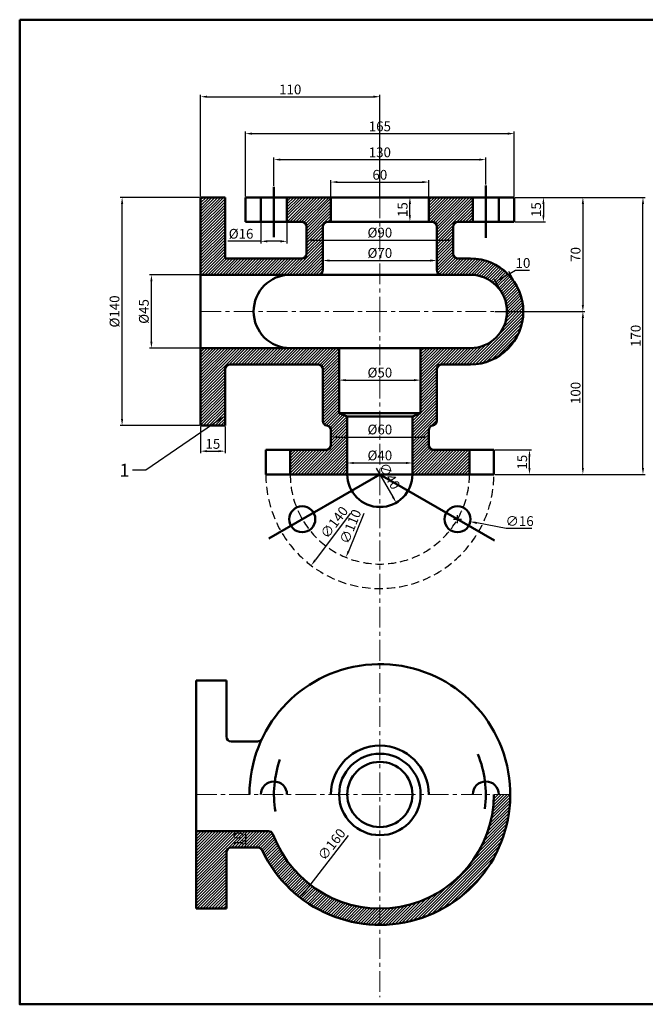
# Model space of a CAD drawing. Units: millimetres. Extents: x -266 to 493, y 251 to 855.
# Tile 1 of 3: x -266 to 118, y 251 to 855. Entities that reach past the tile are written whole.
import ezdxf
from ezdxf import colors
from ezdxf.entities.mleader import LeaderData, LeaderLine
from ezdxf.math import Vec2, Vec3

# ---------------------------------------------------------------- set-up
doc = ezdxf.new("R2010")
doc.units = ezdxf.units.MM
doc.header["$LTSCALE"] = 0.4
doc.linetypes.add('CENTER', pattern=[50.8, 31.75, -6.35, 6.35, -6.35])
doc.linetypes.add('DASHED', pattern=[19.05, 12.7, -6.35])
for name, color, linetype, lineweight in [('M-CNTR', 1, 'CENTER', 18), ('M-DIMS', 2, 'Continuous', 25), ('M-HATC', 8, 'Continuous', 18), ('M-HIDN', 3, 'DASHED', 25), ('M-OUTL', 7, 'Continuous', 50), ('M-TEXT', 7, 'Continuous', 25)]:
    doc.layers.add(name, color=color, linetype=linetype, lineweight=lineweight)
doc.styles.get("Standard").update_dxf_attribs({"font": 'arial.ttf'})
doc.dimstyles.new('ISO-25', dxfattribs={"dimtxt": 6, "dimasz": 4, "dimexe": 1.25, "dimexo": 0.625, "dimtad": 1, "dimtoh": 1, "dimtxsty": 'Standard', "dimcen": 2.5, "dimadec": 0, "dimazin": 0, "dimtfac": 1, "dimtofl": 0, "dimtmove": 0, "dimatfit": 3, "dimfxl": 1, "dimarcsym": 0})

# ---------------------------------------------------------------- blocks, each defined once
blk = doc.blocks.new('*D1')
at = {"layer": 'Defpoints', "color": 0, "transparency": 16777216}
for p in [(-2.49, 631.82), (-86.83, 520.08)]:
    blk.add_point(p, dxfattribs=at)
at = {"layer": 'M-DIMS', "color": 0, "lineweight": -2, "transparency": 16777216}
blk.add_line((-62.64, 552.13), (-84.42, 523.27), dxfattribs=at)
at = {"layer": 'M-DIMS', "color": 0, "transparency": 16777216}
blk.add_solid([(-84.95, 523.68), (-83.89, 522.87), (-86.83, 520.08)], dxfattribs=at)
at = {"layer": 'M-DIMS', "color": 0, "transparency": 16777216, "insert": (-72.05, 546.07), "char_height": 6, "attachment_point": 5, "rotation": 52.95454}
blk.add_mtext('∅140', dxfattribs=at)
blk = doc.blocks.new('*D2')
at = {"layer": 'Defpoints', "color": 0, "transparency": 16777216}
for p in [(-23.86, 626.87), (-65.45, 525.03)]:
    blk.add_point(p, dxfattribs=at)
at = {"layer": 'M-DIMS', "color": 0, "lineweight": -2, "transparency": 16777216}
blk.add_line((-54.48, 551.9), (-63.94, 528.74), dxfattribs=at)
at = {"layer": 'M-DIMS', "color": 0, "transparency": 16777216}
blk.add_solid([(-64.55, 528.99), (-63.32, 528.49), (-65.45, 525.03)], dxfattribs=at)
at = {"layer": 'M-DIMS', "color": 0, "transparency": 16777216, "insert": (-62.02, 543.63), "char_height": 6, "attachment_point": 5, "rotation": 67.78768}
blk.add_mtext('∅110', dxfattribs=at)
blk = doc.blocks.new('*D3')
at = {"layer": 'Defpoints', "color": 0, "transparency": 16777216}
for p in [(-54.66, 593.27), (-34.65, 558.64)]:
    blk.add_point(p, dxfattribs=at)
at = {"layer": 'M-DIMS', "color": 0, "lineweight": -2, "transparency": 16777216}
blk.add_line((-46.83, 579.72), (-36.65, 562.1), dxfattribs=at)
at = {"layer": 'M-DIMS', "color": 0, "transparency": 16777216}
blk.add_solid([(-36.07, 562.43), (-37.23, 561.77), (-34.65, 558.64)], dxfattribs=at)
at = {"layer": 'M-DIMS', "color": 0, "transparency": 16777216, "insert": (-39.4, 574.57), "char_height": 6, "attachment_point": 5, "rotation": 300.02397}
blk.add_mtext('∅40', dxfattribs=at)
blk = doc.blocks.new('*D4')
at = {"layer": 'Defpoints', "color": 0, "transparency": 16777216}
for p in [(-4.88, 549.97), (10.83, 546.93)]:
    blk.add_point(p, dxfattribs=at)
at = {"layer": 'M-DIMS', "color": 0, "lineweight": -2, "transparency": 16777216}
for p, q in [((2.97, 545.95), (2.97, 550.95)), ((0.47, 548.45), (5.47, 548.45)), ((32.94, 542.66), (14.76, 546.18)), ((48.68, 542.66), (32.94, 542.66))]:
    blk.add_line(p, q, dxfattribs=at)
at = {"layer": 'M-DIMS', "color": 0, "transparency": 16777216}
blk.add_solid([(14.88, 546.83), (14.63, 545.52), (10.83, 546.93)], dxfattribs=at)
at = {"layer": 'M-DIMS', "color": 0, "transparency": 16777216, "insert": (41.12, 546.52), "char_height": 6, "attachment_point": 5}
blk.add_mtext('∅16', dxfattribs=at)
blk = doc.blocks.new('*D5')
at = {"layer": 'Defpoints', "color": 0, "transparency": 16777216}
for p in [(-64.66, 587.3), (-24.66, 587.3), (-24.66, 582.96)]:
    blk.add_point(p, dxfattribs=at)
at = {"layer": 'M-DIMS', "color": 0, "lineweight": -2, "transparency": 16777216}
for p, q in [((-64.66, 586.67), (-64.66, 581.71)), ((-24.66, 586.67), (-24.66, 581.71)), ((-60.66, 582.96), (-28.66, 582.96))]:
    blk.add_line(p, q, dxfattribs=at)
at = {"layer": 'M-DIMS', "color": 0, "transparency": 16777216}
for points in [[(-60.66, 583.63), (-60.66, 582.3), (-64.66, 582.96)], [(-28.66, 583.63), (-28.66, 582.3), (-24.66, 582.96)]]:
    blk.add_solid(points, dxfattribs=at)
at = {"layer": 'M-DIMS', "color": 0, "transparency": 16777216, "insert": (-44.66, 586.82), "char_height": 6, "attachment_point": 5}
blk.add_mtext('%%C40', dxfattribs=at)
blk = doc.blocks.new('*D6')
at = {"layer": 'Defpoints', "color": 0, "transparency": 16777216}
for p in [(-74.66, 598.45), (-14.66, 598.87), (-14.66, 598.45)]:
    blk.add_point(p, dxfattribs=at)
at = {"layer": 'M-DIMS', "color": 0, "lineweight": -2, "transparency": 16777216}
for p, q in [((-74.66, 599.08), (-74.66, 600.12)), ((-70.66, 598.87), (-18.66, 598.87)), ((-14.66, 599.08), (-14.66, 600.12))]:
    blk.add_line(p, q, dxfattribs=at)
at = {"layer": 'M-DIMS', "color": 0, "transparency": 16777216}
for points in [[(-70.66, 599.54), (-70.66, 598.2), (-74.66, 598.87)], [(-18.66, 599.54), (-18.66, 598.2), (-14.66, 598.87)]]:
    blk.add_solid(points, dxfattribs=at)
at = {"layer": 'M-DIMS', "color": 0, "transparency": 16777216, "insert": (-44.66, 602.73), "char_height": 6, "attachment_point": 5}
blk.add_mtext('%%C60', dxfattribs=at)
blk = doc.blocks.new('*D7')
at = {"layer": 'Defpoints', "color": 0, "transparency": 16777216}
for p in [(-69.66, 633.45), (-19.66, 633.8), (-19.66, 633.45)]:
    blk.add_point(p, dxfattribs=at)
at = {"layer": 'M-DIMS', "color": 0, "lineweight": -2, "transparency": 16777216}
for p, q in [((-69.66, 634.08), (-69.66, 635.05)), ((-19.66, 634.08), (-19.66, 635.05)), ((-65.66, 633.8), (-23.66, 633.8))]:
    blk.add_line(p, q, dxfattribs=at)
at = {"layer": 'M-DIMS', "color": 0, "transparency": 16777216}
for points in [[(-65.66, 634.47), (-65.66, 633.14), (-69.66, 633.8)], [(-23.66, 634.47), (-23.66, 633.14), (-19.66, 633.8)]]:
    blk.add_solid(points, dxfattribs=at)
at = {"layer": 'M-DIMS', "color": 0, "transparency": 16777216, "insert": (-44.66, 637.66), "char_height": 6, "attachment_point": 5}
blk.add_mtext('%%C50', dxfattribs=at)
blk = doc.blocks.new('*D8')
at = {"layer": 'Defpoints', "color": 0, "transparency": 16777216}
for p in [(-154.66, 605.95), (-139.66, 605.97), (-139.66, 590.21)]:
    blk.add_point(p, dxfattribs=at)
at = {"layer": 'M-DIMS', "color": 0, "lineweight": -2, "transparency": 16777216}
for p, q in [((-154.66, 605.33), (-154.66, 588.96)), ((-139.66, 605.34), (-139.66, 588.96)), ((-150.66, 590.21), (-143.66, 590.21))]:
    blk.add_line(p, q, dxfattribs=at)
at = {"layer": 'M-DIMS', "color": 0, "transparency": 16777216}
for points in [[(-150.66, 590.88), (-150.66, 589.55), (-154.66, 590.21)], [(-143.66, 590.88), (-143.66, 589.55), (-139.66, 590.21)]]:
    blk.add_solid(points, dxfattribs=at)
at = {"layer": 'M-DIMS', "color": 0, "transparency": 16777216, "insert": (-147.16, 593.9), "char_height": 6, "attachment_point": 5}
blk.add_mtext('15', dxfattribs=at)
blk = doc.blocks.new('*D9')
at = {"layer": 'Defpoints', "color": 0, "transparency": 16777216}
for p in [(25.34, 590.95), (47.16, 590.95), (25.34, 575.95)]:
    blk.add_point(p, dxfattribs=at)
at = {"layer": 'M-DIMS', "color": 0, "lineweight": -2, "transparency": 16777216}
for p, q in [((25.97, 590.95), (48.41, 590.95)), ((47.16, 579.95), (47.16, 586.95)), ((25.97, 575.95), (48.41, 575.95))]:
    blk.add_line(p, q, dxfattribs=at)
at = {"layer": 'M-DIMS', "color": 0, "transparency": 16777216}
for points in [[(46.5, 586.95), (47.83, 586.95), (47.16, 590.95)], [(46.5, 579.95), (47.83, 579.95), (47.16, 575.95)]]:
    blk.add_solid(points, dxfattribs=at)
at = {"layer": 'M-DIMS', "color": 0, "transparency": 16777216, "insert": (43.47, 583.45), "char_height": 6, "attachment_point": 5, "rotation": 90}
blk.add_mtext('15', dxfattribs=at)
blk = doc.blocks.new('*D10')
at = {"layer": 'Defpoints', "color": 0, "transparency": 16777216}
for p in [(-202.86, 745.95), (-154.66, 745.95), (-154.66, 605.95)]:
    blk.add_point(p, dxfattribs=at)
at = {"layer": 'M-DIMS', "color": 0, "lineweight": -2, "transparency": 16777216}
for p, q in [((-155.28, 745.95), (-204.11, 745.95)), ((-202.86, 609.95), (-202.86, 741.95)), ((-155.28, 605.95), (-204.11, 605.95))]:
    blk.add_line(p, q, dxfattribs=at)
at = {"layer": 'M-DIMS', "color": 0, "transparency": 16777216}
for points in [[(-203.53, 741.95), (-202.19, 741.95), (-202.86, 745.95)], [(-203.53, 609.95), (-202.19, 609.95), (-202.86, 605.95)]]:
    blk.add_solid(points, dxfattribs=at)
at = {"layer": 'M-DIMS', "color": 0, "transparency": 16777216, "insert": (-206.72, 675.95), "char_height": 6, "attachment_point": 5, "rotation": 90}
blk.add_mtext('%%C140', dxfattribs=at)
blk = doc.blocks.new('*D11')
at = {"layer": 'Defpoints', "color": 0, "transparency": 16777216}
for p in [(-184.87, 698.45), (-154.66, 698.45), (-154.66, 653.45)]:
    blk.add_point(p, dxfattribs=at)
at = {"layer": 'M-DIMS', "color": 0, "lineweight": -2, "transparency": 16777216}
for p, q in [((-155.28, 698.45), (-186.12, 698.45)), ((-184.87, 657.45), (-184.87, 694.45)), ((-155.28, 653.45), (-186.12, 653.45))]:
    blk.add_line(p, q, dxfattribs=at)
at = {"layer": 'M-DIMS', "color": 0, "transparency": 16777216}
for points in [[(-185.54, 694.45), (-184.2, 694.45), (-184.87, 698.45)], [(-185.54, 657.45), (-184.2, 657.45), (-184.87, 653.45)]]:
    blk.add_solid(points, dxfattribs=at)
at = {"layer": 'M-DIMS', "color": 0, "transparency": 16777216, "insert": (-188.73, 675.95), "char_height": 6, "attachment_point": 5, "rotation": 90}
blk.add_mtext('%%C45', dxfattribs=at)
blk = doc.blocks.new('*D12')
at = {"layer": 'Defpoints', "color": 0, "transparency": 16777216}
for p in [(37.84, 745.95), (116.82, 745.95), (25.34, 575.95)]:
    blk.add_point(p, dxfattribs=at)
at = {"layer": 'M-DIMS', "color": 0, "lineweight": -2, "transparency": 16777216}
for p, q in [((38.47, 745.95), (118.07, 745.95)), ((116.82, 579.95), (116.82, 741.95)), ((25.97, 575.95), (118.07, 575.95))]:
    blk.add_line(p, q, dxfattribs=at)
at = {"layer": 'M-DIMS', "color": 0, "transparency": 16777216}
for points in [[(116.15, 741.95), (117.48, 741.95), (116.82, 745.95)], [(116.15, 579.95), (117.48, 579.95), (116.82, 575.95)]]:
    blk.add_solid(points, dxfattribs=at)
at = {"layer": 'M-DIMS', "color": 0, "transparency": 16777216, "insert": (113.13, 660.95), "char_height": 6, "attachment_point": 5, "rotation": 90}
blk.add_mtext('170', dxfattribs=at)
blk = doc.blocks.new('*D13')
at = {"layer": 'Defpoints', "color": 0, "transparency": 16777216}
for p in [(25.34, 675.95), (79.94, 675.95), (25.34, 575.95)]:
    blk.add_point(p, dxfattribs=at)
at = {"layer": 'M-DIMS', "color": 0, "lineweight": -2, "transparency": 16777216}
for p, q in [((25.97, 675.95), (81.19, 675.95)), ((79.94, 579.95), (79.94, 671.95)), ((25.97, 575.95), (81.19, 575.95))]:
    blk.add_line(p, q, dxfattribs=at)
at = {"layer": 'M-DIMS', "color": 0, "transparency": 16777216}
for points in [[(79.27, 671.95), (80.61, 671.95), (79.94, 675.95)], [(79.27, 579.95), (80.61, 579.95), (79.94, 575.95)]]:
    blk.add_solid(points, dxfattribs=at)
at = {"layer": 'M-DIMS', "color": 0, "transparency": 16777216, "insert": (76.25, 625.95), "char_height": 6, "attachment_point": 5, "rotation": 90}
blk.add_mtext('100', dxfattribs=at)
blk = doc.blocks.new('*D14')
at = {"layer": 'Defpoints', "color": 0, "transparency": 16777216}
for p in [(37.84, 745.95), (37.84, 675.95), (79.94, 675.95)]:
    blk.add_point(p, dxfattribs=at)
at = {"layer": 'M-DIMS', "color": 0, "lineweight": -2, "transparency": 16777216}
for p, q in [((38.47, 745.95), (81.19, 745.95)), ((79.94, 741.95), (79.94, 679.95)), ((38.47, 675.95), (81.19, 675.95))]:
    blk.add_line(p, q, dxfattribs=at)
at = {"layer": 'M-DIMS', "color": 0, "transparency": 16777216}
for points in [[(79.27, 741.95), (80.61, 741.95), (79.94, 745.95)], [(79.27, 679.95), (80.61, 679.95), (79.94, 675.95)]]:
    blk.add_solid(points, dxfattribs=at)
at = {"layer": 'M-DIMS', "color": 0, "transparency": 16777216, "insert": (76.25, 710.95), "char_height": 6, "attachment_point": 5, "rotation": 90}
blk.add_mtext('70', dxfattribs=at)
blk = doc.blocks.new('*D15')
at = {"layer": 'Defpoints', "color": 0, "transparency": 16777216}
for p in [(37.84, 745.95), (37.84, 730.95), (55.71, 730.95)]:
    blk.add_point(p, dxfattribs=at)
at = {"layer": 'M-DIMS', "color": 0, "lineweight": -2, "transparency": 16777216}
for p, q in [((38.47, 745.95), (56.96, 745.95)), ((55.71, 741.95), (55.71, 734.95)), ((38.47, 730.95), (56.96, 730.95))]:
    blk.add_line(p, q, dxfattribs=at)
at = {"layer": 'M-DIMS', "color": 0, "transparency": 16777216}
for points in [[(55.05, 741.95), (56.38, 741.95), (55.71, 745.95)], [(55.05, 734.95), (56.38, 734.95), (55.71, 730.95)]]:
    blk.add_solid(points, dxfattribs=at)
at = {"layer": 'M-DIMS', "color": 0, "transparency": 16777216, "insert": (52.02, 738.45), "char_height": 6, "attachment_point": 5, "rotation": 90}
blk.add_mtext('15', dxfattribs=at)
blk = doc.blocks.new('*D16')
at = {"layer": 'Defpoints', "color": 0, "transparency": 16777216}
for p in [(35.05, 699.28), (39.23, 691.82), (30.5, 686.94)]:
    blk.add_point(p, dxfattribs=at)
at = {"layer": 'M-DIMS', "color": 0, "lineweight": -2, "transparency": 16777216}
for p, q in [((35.05, 699.28), (38.54, 701.24)), ((38.54, 701.24), (47.18, 701.24)), ((30.2, 687.48), (25.72, 695.49)), ((29.82, 696.35), (31.56, 697.33)), ((38.92, 692.37), (34.44, 700.37))]:
    blk.add_line(p, q, dxfattribs=at)
at = {"layer": 'M-DIMS', "color": 0, "transparency": 16777216}
for points in [[(29.49, 696.94), (30.14, 695.77), (26.33, 694.4)], [(31.24, 697.91), (31.89, 696.75), (35.05, 699.28)]]:
    blk.add_solid(points, dxfattribs=at)
at = {"layer": 'M-DIMS', "color": 0, "transparency": 16777216, "insert": (43.17, 704.93), "char_height": 6, "attachment_point": 5}
blk.add_mtext('10', dxfattribs=at)
blk = doc.blocks.new('*D17')
at = {"layer": 'Defpoints', "color": 0, "transparency": 16777216}
for p in [(-79.66, 714.7), (-9.66, 714.7), (-9.66, 707.2)]:
    blk.add_point(p, dxfattribs=at)
at = {"layer": 'M-DIMS', "color": 0, "lineweight": -2, "transparency": 16777216}
for p, q in [((-79.66, 714.08), (-79.66, 705.95)), ((-9.66, 714.08), (-9.66, 705.95)), ((-75.66, 707.2), (-13.66, 707.2))]:
    blk.add_line(p, q, dxfattribs=at)
at = {"layer": 'M-DIMS', "color": 0, "transparency": 16777216}
for points in [[(-75.66, 707.87), (-75.66, 706.54), (-79.66, 707.2)], [(-13.66, 707.87), (-13.66, 706.54), (-9.66, 707.2)]]:
    blk.add_solid(points, dxfattribs=at)
at = {"layer": 'M-DIMS', "color": 0, "transparency": 16777216, "insert": (-44.66, 711.06), "char_height": 6, "attachment_point": 5}
blk.add_mtext('%%C70', dxfattribs=at)
blk = doc.blocks.new('*D18')
at = {"layer": 'Defpoints', "color": 0, "transparency": 16777216}
for p in [(-89.66, 719.7), (0.34, 719.7), (0.34, 719.7)]:
    blk.add_point(p, dxfattribs=at)
at = {"layer": 'M-DIMS', "color": 0, "lineweight": -2, "transparency": 16777216}
for p, q in [((-89.66, 720.33), (-89.66, 720.95)), ((-85.66, 719.7), (-3.66, 719.7)), ((0.34, 720.33), (0.34, 720.95))]:
    blk.add_line(p, q, dxfattribs=at)
at = {"layer": 'M-DIMS', "color": 0, "transparency": 16777216}
for points in [[(-85.66, 720.37), (-85.66, 719.04), (-89.66, 719.7)], [(-3.66, 720.37), (-3.66, 719.04), (0.34, 719.7)]]:
    blk.add_solid(points, dxfattribs=at)
at = {"layer": 'M-DIMS', "color": 0, "transparency": 16777216, "insert": (-44.66, 723.56), "char_height": 6, "attachment_point": 5}
blk.add_mtext('%%C90', dxfattribs=at)
blk = doc.blocks.new('*D19')
at = {"layer": 'Defpoints', "color": 0, "transparency": 16777216}
for p in [(-14.66, 755.34), (-74.66, 745.95), (-14.66, 745.95)]:
    blk.add_point(p, dxfattribs=at)
at = {"layer": 'M-DIMS', "color": 0, "lineweight": -2, "transparency": 16777216}
for p, q in [((-74.66, 746.58), (-74.66, 756.59)), ((-70.66, 755.34), (-18.66, 755.34)), ((-14.66, 746.58), (-14.66, 756.59))]:
    blk.add_line(p, q, dxfattribs=at)
at = {"layer": 'M-DIMS', "color": 0, "transparency": 16777216}
for points in [[(-70.66, 756.01), (-70.66, 754.68), (-74.66, 755.34)], [(-18.66, 756.01), (-18.66, 754.68), (-14.66, 755.34)]]:
    blk.add_solid(points, dxfattribs=at)
at = {"layer": 'M-DIMS', "color": 0, "transparency": 16777216, "insert": (-44.66, 759.03), "char_height": 6, "attachment_point": 5}
blk.add_mtext('60', dxfattribs=at)
blk = doc.blocks.new('*D20')
at = {"layer": 'Defpoints', "color": 0, "transparency": 16777216}
for p in [(20.34, 769.13), (-109.66, 752.41), (20.34, 753.27)]:
    blk.add_point(p, dxfattribs=at)
at = {"layer": 'M-DIMS', "color": 0, "lineweight": -2, "transparency": 16777216}
for p, q in [((-109.66, 753.03), (-109.66, 770.38)), ((-105.66, 769.13), (16.34, 769.13)), ((20.34, 753.9), (20.34, 770.38))]:
    blk.add_line(p, q, dxfattribs=at)
at = {"layer": 'M-DIMS', "color": 0, "transparency": 16777216}
for points in [[(-105.66, 769.8), (-105.66, 768.47), (-109.66, 769.13)], [(16.34, 769.8), (16.34, 768.47), (20.34, 769.13)]]:
    blk.add_solid(points, dxfattribs=at)
at = {"layer": 'M-DIMS', "color": 0, "transparency": 16777216, "insert": (-44.66, 772.82), "char_height": 6, "attachment_point": 5}
blk.add_mtext('130', dxfattribs=at)
blk = doc.blocks.new('*D21')
at = {"layer": 'Defpoints', "color": 0, "transparency": 16777216}
for p in [(37.84, 785.08), (-127.16, 745.95), (37.84, 745.95)]:
    blk.add_point(p, dxfattribs=at)
at = {"layer": 'M-DIMS', "color": 0, "lineweight": -2, "transparency": 16777216}
for p, q in [((-127.16, 746.58), (-127.16, 786.33)), ((37.84, 746.58), (37.84, 786.33)), ((-123.16, 785.08), (33.84, 785.08))]:
    blk.add_line(p, q, dxfattribs=at)
at = {"layer": 'M-DIMS', "color": 0, "transparency": 16777216}
for points in [[(-123.16, 785.74), (-123.16, 784.41), (-127.16, 785.08)], [(33.84, 785.74), (33.84, 784.41), (37.84, 785.08)]]:
    blk.add_solid(points, dxfattribs=at)
at = {"layer": 'M-DIMS', "color": 0, "transparency": 16777216, "insert": (-44.66, 788.77), "char_height": 6, "attachment_point": 5}
blk.add_mtext('165', dxfattribs=at)
blk = doc.blocks.new('*D22')
at = {"layer": 'Defpoints', "color": 0, "transparency": 16777216}
for p in [(-44.66, 807.72), (-154.66, 745.95), (-44.66, 745.95)]:
    blk.add_point(p, dxfattribs=at)
at = {"layer": 'M-DIMS', "color": 0, "lineweight": -2, "transparency": 16777216}
for p, q in [((-154.66, 746.58), (-154.66, 808.97)), ((-150.66, 807.72), (-48.66, 807.72)), ((-44.66, 746.58), (-44.66, 808.97))]:
    blk.add_line(p, q, dxfattribs=at)
at = {"layer": 'M-DIMS', "color": 0, "transparency": 16777216}
for points in [[(-150.66, 808.39), (-150.66, 807.06), (-154.66, 807.72)], [(-48.66, 808.39), (-48.66, 807.06), (-44.66, 807.72)]]:
    blk.add_solid(points, dxfattribs=at)
at = {"layer": 'M-DIMS', "color": 0, "transparency": 16777216, "insert": (-99.66, 811.41), "char_height": 6, "attachment_point": 5}
blk.add_mtext('110', dxfattribs=at)
blk = doc.blocks.new('*D23')
at = {"layer": 'Defpoints', "color": 0, "transparency": 16777216}
for p in [(-117.66, 730.95), (-101.66, 730.95), (-101.66, 718.99)]:
    blk.add_point(p, dxfattribs=at)
at = {"layer": 'M-DIMS', "color": 0, "lineweight": -2, "transparency": 16777216}
for p, q in [((-117.66, 730.33), (-117.66, 717.74)), ((-101.66, 730.33), (-101.66, 717.74)), ((-117.66, 718.99), (-138.03, 718.99)), ((-105.66, 718.99), (-113.66, 718.99))]:
    blk.add_line(p, q, dxfattribs=at)
at = {"layer": 'M-DIMS', "color": 0, "transparency": 16777216}
for points in [[(-113.66, 719.66), (-113.66, 718.32), (-117.66, 718.99)], [(-105.66, 719.66), (-105.66, 718.32), (-101.66, 718.99)]]:
    blk.add_solid(points, dxfattribs=at)
at = {"layer": 'M-DIMS', "color": 0, "transparency": 16777216, "insert": (-129.84, 722.84), "char_height": 6, "attachment_point": 5}
blk.add_mtext('%%C16', dxfattribs=at)
blk = doc.blocks.new('*D24')
at = {"layer": 'Defpoints', "color": 0, "transparency": 16777216}
for p in [(-26.23, 745.95), (-23.61, 745.95), (-23.61, 730.95)]:
    blk.add_point(p, dxfattribs=at)
at = {"layer": 'M-DIMS', "color": 0, "lineweight": -2, "transparency": 16777216}
for p, q in [((-24.24, 745.95), (-27.48, 745.95)), ((-26.23, 734.95), (-26.23, 741.95)), ((-24.24, 730.95), (-27.48, 730.95))]:
    blk.add_line(p, q, dxfattribs=at)
at = {"layer": 'M-DIMS', "color": 0, "transparency": 16777216}
for points in [[(-26.9, 741.95), (-25.57, 741.95), (-26.23, 745.95)], [(-26.9, 734.95), (-25.57, 734.95), (-26.23, 730.95)]]:
    blk.add_solid(points, dxfattribs=at)
at = {"layer": 'M-DIMS', "color": 0, "transparency": 16777216, "insert": (-29.92, 738.45), "char_height": 6, "attachment_point": 5, "rotation": 90}
blk.add_mtext('15', dxfattribs=at)
blk = doc.blocks.new('*D25')
at = {"layer": 'Defpoints', "color": 0, "transparency": 16777216}
for p in [(4.35, 442.79), (-93.66, 316.32)]:
    blk.add_point(p, dxfattribs=at)
at = {"layer": 'M-DIMS', "color": 0, "lineweight": -2, "transparency": 16777216}
blk.add_line((-64.16, 354.38), (-91.21, 319.48), dxfattribs=at)
at = {"layer": 'M-DIMS', "color": 0, "transparency": 16777216}
blk.add_solid([(-91.74, 319.89), (-90.68, 319.07), (-93.66, 316.32)], dxfattribs=at)
at = {"layer": 'M-DIMS', "color": 0, "transparency": 16777216, "insert": (-73.65, 348.44), "char_height": 6, "attachment_point": 5, "rotation": 52.22465}
blk.add_mtext('∅160', dxfattribs=at)
blk = doc.blocks.new('*D26')
at = {"layer": 'Defpoints', "color": 0, "transparency": 16777216}
for p in [(-129.86, 357.05), (-129.86, 347.05), (-127.02, 347.05)]:
    blk.add_point(p, dxfattribs=at)
at = {"layer": 'M-DIMS', "color": 0, "lineweight": -2, "transparency": 16777216}
for p, q in [((-129.24, 357.05), (-125.77, 357.05)), ((-127.02, 353.05), (-127.02, 351.05)), ((-129.24, 347.05), (-125.77, 347.05))]:
    blk.add_line(p, q, dxfattribs=at)
at = {"layer": 'M-DIMS', "color": 0, "transparency": 16777216}
for points in [[(-127.69, 353.05), (-126.36, 353.05), (-127.02, 357.05)], [(-127.69, 351.05), (-126.36, 351.05), (-127.02, 347.05)]]:
    blk.add_solid(points, dxfattribs=at)
at = {"layer": 'M-DIMS', "color": 0, "transparency": 16777216, "insert": (-130.71, 352.05), "char_height": 6, "attachment_point": 5, "rotation": 90}
blk.add_mtext('10', dxfattribs=at)

msp = doc.modelspace()

# ---------------------------------------------------------------- hatches: boundary and pattern name
at = {"layer": 'M-HATC', "ltscale": 0.4}
h = msp.add_hatch(dxfattribs=at)
h.set_pattern_fill('ANSI31', color=256, scale=0.4)
h.set_pattern_definition([(45, (-492.9546, -138.1021), (-0.8980256, 0.8980256), [])])
h.paths.add_polyline_path([(-154.657, 605.953), (-139.657, 605.969), (-139.657, 640.453, -0.4142136), (-136.657, 643.453), (-82.657, 643.453, -0.4142136), (-79.657, 640.453), (-79.657, 608.869, 0.3659774), (-77.157, 605.911, -0.3659774), (-74.657, 602.953), (-74.657, 593.953, -0.4142136), (-77.657, 590.953), (-99.657, 590.953), (-99.657, 575.953), (-64.657, 575.953), (-64.657, 611.453), (-69.657, 613.453), (-69.657, 653.453), (-154.657, 653.453)])
h.paths.add_polyline_path([(-9.657, 640.453, -0.4142136), (-6.657, 643.453), (10.866, 643.453, 1), (10.866, 708.453), (3.343, 708.453, -0.4142136), (0.343, 711.453), (0.343, 727.953, -0.4142136), (3.343, 730.953), (12.343, 730.953), (12.343, 745.953), (-14.657, 745.953), (-14.657, 730.953), (-12.657, 730.953, -0.4142136), (-9.657, 727.953), (-9.657, 701.453, 0.4142136), (-6.657, 698.453), (10.866, 698.453, -1), (10.866, 653.453), (-19.657, 653.453), (-19.657, 613.453), (-24.657, 611.453), (-24.657, 575.953), (10.343, 575.953), (10.343, 590.953), (-11.657, 590.953, -0.4142136), (-14.657, 593.953), (-14.657, 603.104, -0.3659774), (-12.157, 606.062, 0.3659774), (-9.657, 609.02)])
h.paths.add_polyline_path([(-101.657, 745.953), (-101.657, 730.953), (-92.657, 730.953, -0.4142136), (-89.657, 727.953), (-89.657, 711.453, -0.4142136), (-92.657, 708.453), (-139.657, 708.453), (-139.657, 745.953), (-154.657, 745.953), (-154.657, 698.453), (-82.657, 698.453, 0.4142136), (-79.657, 701.453), (-79.657, 727.953, -0.4142136), (-76.657, 730.953), (-74.657, 730.953), (-74.657, 745.953)])
h.paths.add_polyline_path([(36.756, 698.688), (49.079, 698.688), (49.079, 711.052), (36.756, 711.052)], flags=9)
at = {"layer": 'M-HATC'}
h = msp.add_hatch(dxfattribs=at)
h.set_pattern_fill('ANSI31', color=256, scale=0.4)
h.set_pattern_definition([(45, (-780.3092, -105.4534), (-0.8980256, 0.8980256), [])])
h.paths.add_polyline_path([(-110.247, 355.101, 0.3131633), (-113.058, 357.053), (-157.42, 357.053), (-157.42, 309.553), (-138.881, 309.553), (-138.881, 344.053, -0.4142136), (-135.881, 347.053), (-119.682, 347.053, -0.2899479), (-116.97, 345.336, 0.2899479), (-44.657, 299.553), (-44.657, 309.553, -0.3131633)])
h.paths.add_polyline_path([(35.343, 379.553), (25.343, 379.553, -0.4142136), (-44.657, 309.553), (-44.657, 299.553, 0.4142136)])

# ---------------------------------------------------------------- linework, layer by layer
at = {"layer": 'M-CNTR'}
for p, q in [((-154.657, 675.953), (25.343, 675.953)), ((-157.42, 379.553), (35.343, 379.553))]:
    msp.add_line(p, q, dxfattribs=at)
msp.add_lwpolyline([(-44.657, 745.953), (-44.657, 675.953), (-44.657, 575.953), (-44.657, 255.246)], dxfattribs=at)
at = {"layer": 'M-HIDN'}
for radius in [70, 55]:
    msp.add_arc((-44.657, 575.953), radius, 180, 0, dxfattribs=at)
at = {"layer": 'M-OUTL'}
for p, q in [((-109.657, 752.409), (-109.657, 721.437)), ((20.343, 753.275), (20.343, 721.091)), ((-154.657, 745.953), (-139.657, 745.953)), ((-154.657, 745.953), (-154.657, 605.953)), ((-139.657, 708.453), (-139.657, 745.953)), ((-127.157, 745.953), (-127.157, 730.953)), ((-127.157, 745.953), (25.343, 745.953)), ((-117.657, 745.953), (-117.657, 730.953)), ((-114.657, 745.953), (25.343, 745.953)), ((-114.657, 745.953), (25.343, 745.953)), ((-114.657, 745.953), (37.843, 745.953)), ((-101.657, 745.953), (-101.657, 730.953)), ((-74.657, 745.953), (-74.657, 730.953)), ((-14.657, 745.953), (-14.657, 730.953)), ((12.343, 745.953), (12.343, 730.953)), ((28.343, 745.953), (28.343, 730.953)), ((37.843, 745.953), (37.843, 730.953)), ((-127.157, 730.953), (-92.657, 730.953)), ((-89.657, 727.953), (-89.657, 711.453)), ((-79.657, 727.953), (-79.657, 701.453)), ((-76.657, 730.953), (-12.657, 730.953)), ((-9.657, 727.953), (-9.657, 701.453)), ((0.343, 727.953), (0.343, 711.453)), ((3.343, 730.953), (37.843, 730.953)), ((-139.657, 708.453), (-92.657, 708.453)), ((3.343, 708.453), (10.866, 708.453)), ((-154.657, 698.453), (-82.657, 698.453)), ((-82.657, 698.453), (-6.657, 698.453)), ((-6.657, 698.453), (10.866, 698.453)), ((-154.657, 653.453), (10.866, 653.453)), ((-69.657, 653.453), (-69.657, 613.453)), ((-19.657, 653.453), (-19.657, 613.453)), ((-136.657, 643.453), (-82.657, 643.453)), ((-6.657, 643.453), (10.866, 643.453)), ((-139.657, 605.969), (-139.657, 640.453)), ((-79.657, 640.453), (-79.657, 608.869)), ((-9.657, 640.453), (-9.657, 609.02)), ((-69.657, 613.453), (-19.657, 613.453)), ((-64.657, 611.453), (-69.657, 613.453)), ((-64.657, 611.453), (-24.657, 611.453)), ((-64.657, 611.453), (-64.657, 575.953)), ((-24.657, 611.453), (-19.657, 613.453)), ((-24.657, 611.453), (-24.657, 575.953)), ((-154.657, 605.953), (-139.657, 605.969)), ((-74.657, 602.953), (-74.657, 593.953)), ((-14.657, 603.104), (-14.657, 593.953)), ((-114.657, 590.953), (-114.657, 575.953)), ((-77.657, 590.953), (-114.657, 590.953)), ((-99.657, 590.953), (-99.657, 575.953)), ((25.343, 590.953), (-11.657, 590.953)), ((10.343, 575.953), (10.343, 590.953)), ((25.343, 575.953), (25.343, 590.953)), ((-114.657, 575.953), (25.343, 575.953)), ((-44.657, 575.953), (-112.867, 536.571)), ((-44.657, 575.953), (25.643, 535.365)), ((-157.42, 449.553), (-138.881, 449.553)), ((-157.42, 449.553), (-157.42, 309.553)), ((-138.881, 449.553), (-138.881, 415.053)), ((-135.881, 412.053), (-119.682, 412.053)), ((-157.42, 357.053), (-113.058, 357.053)), ((-135.881, 347.053), (-119.682, 347.053)), ((-138.881, 344.053), (-138.881, 309.553)), ((-157.42, 309.553), (-138.881, 309.553))]:
    msp.add_line(p, q, dxfattribs=at)
at = {"layer": 'M-OUTL', "ltscale": 0.4}
msp.add_lwpolyline([(-265.707, 854.992), (492.506, 854.992), (492.506, 250.777), (-265.707, 250.777)], close=True, dxfattribs=at)
at = {"layer": 'M-OUTL'}
for centre, radius in [((-92.288, 548.453), 8), ((2.975, 548.453), 8), ((-44.657, 379.553), 25), ((-44.657, 379.553), 20)]:
    msp.add_circle(centre, radius, dxfattribs=at)
for centre, radius, start, end in [((-92.657, 727.953), 3, 0, 90), ((-76.657, 727.953), 3, 90, 180), ((-12.657, 727.953), 3, 0, 90), ((3.343, 727.953), 3, 90, 180), ((-92.657, 711.453), 3, 270, 0), ((3.343, 711.453), 3, 180, 270), ((10.866, 675.953), 32.5, 270, 90), ((-82.657, 701.453), 3, 270, 0), ((-6.657, 701.453), 3, 180, 185.512583), ((-6.657, 701.453), 3, 180, 270), ((-99.657, 675.953), 22.5, 90, 270), ((10.866, 675.953), 22.5, 270, 90), ((-136.657, 640.453), 3, 90, 180), ((-82.657, 640.453), 3, 0, 90), ((-6.657, 640.453), 3, 90, 180), ((-76.657, 608.869), 3, 180, 260.405932), ((-77.657, 602.953), 3, 0, 80.405932), ((-11.657, 603.104), 3, 99.594068, 180), ((-12.657, 609.02), 3, 279.594068, 0), ((-77.657, 593.953), 3, 270, 0), ((-11.657, 593.953), 3, 180, 270), ((-44.657, 575.953), 20, 180, 0), ((-44.657, 379.553), 80, 205.322372, 180), ((-135.881, 415.053), 3, 180, 270), ((-119.682, 415.053), 3, 270, 334.677628), ((-44.657, 379.553), 30, 0, 180), ((-44.657, 379.553), 65, 160.6504, 189.253405), ((-44.657, 379.553), 65, 352.272756, 22.284131), ((-109.657, 379.553), 8, 0, 180), ((20.343, 379.553), 8, 0, 180), ((-44.657, 379.553), 70, 200.445427, 0), ((-113.058, 354.053), 3, 20.445427, 90), ((-135.881, 344.053), 3, 90, 180), ((-119.682, 344.053), 3, 25.322372, 90)]:
    msp.add_arc(centre, radius, start, end, dxfattribs=at)

# ---------------------------------------------------------------- dimensions: what is measured, and where the dimension line sits
at = {"layer": 'M-DIMS'}
for base, p1, p2, picture, middle in [((-44.657, 807.722), (-154.657, 745.953), (-44.657, 745.953), '*D22', (-99.657, 811.411)), ((37.843, 785.077), (-127.157, 745.953), (37.843, 745.953), '*D21', (-44.657, 788.766)), ((20.343, 769.133), (-109.657, 752.409), (20.343, 753.275), '*D20', (-44.657, 772.824)), ((-14.657, 755.342), (-74.657, 745.953), (-14.657, 745.953), '*D19', (-44.657, 759.031)), ((-139.657, 590.214), (-154.657, 605.953), (-139.657, 605.969), '*D8', (-147.157, 593.902))]:
    dim = msp.add_linear_dim(base=base, p1=p1, p2=p2, dimstyle='ISO-25', override={"dimclrd": 0, "dimclre": 0, "dimclrt": 0}, dxfattribs=at)
    dim.commit()
    dim.dimension.update_dxf_attribs({"geometry": picture, "text_midpoint": middle})
dim = msp.add_linear_dim(base=(-202.86, 745.953), p1=(-154.657, 605.953), p2=(-154.657, 745.953), angle=90, text='%%C<>', dimstyle='ISO-25', override={"dimclrd": 0, "dimclre": 0, "dimclrt": 0}, dxfattribs=at)
dim.commit()
dim.dimension.update_dxf_attribs({"geometry": '*D10', "text_midpoint": (-202.86, 675.953), "dimtype": 160})
for base, p1, p2, picture, middle in [((-26.234, 745.953), (-23.612, 730.953), (-23.612, 745.953), '*D24', (-29.923, 738.453)), ((116.816, 745.953), (25.343, 575.953), (37.843, 745.953), '*D12', (113.127, 660.953)), ((79.939, 675.953), (37.843, 745.953), (37.843, 675.953), '*D14', (76.251, 710.953)), ((55.712, 730.953), (37.843, 745.953), (37.843, 730.953), '*D15', (52.024, 738.453)), ((79.939, 675.953), (25.343, 575.953), (25.343, 675.953), '*D13', (76.251, 625.953)), ((47.163, 590.953), (25.343, 575.953), (25.343, 590.953), '*D9', (43.474, 583.453))]:
    dim = msp.add_linear_dim(base=base, p1=p1, p2=p2, angle=90, dimstyle='ISO-25', override={"dimclrd": 0, "dimclre": 0, "dimclrt": 0}, dxfattribs=at)
    dim.commit()
    dim.dimension.update_dxf_attribs({"geometry": picture, "text_midpoint": middle})
for base, p1, p2, picture, middle in [((-101.657, 718.989), (-117.657, 730.953), (-101.657, 730.953), '*D23', (-129.841, 718.989)), ((-9.657, 707.203), (-79.657, 714.703), (-9.657, 714.703), '*D17', (-44.657, 707.203))]:
    dim = msp.add_linear_dim(base=base, p1=p1, p2=p2, text='%%C<>', dimstyle='ISO-25', override={"dimclrd": 0, "dimclre": 0, "dimclrt": 0}, dxfattribs=at)
    dim.commit()
    dim.dimension.update_dxf_attribs({"geometry": picture, "text_midpoint": middle, "dimtype": 160})
for base, p1, p2, picture, middle in [((0.343, 719.703), (-89.657, 719.703), (0.343, 719.703), '*D18', (-44.657, 723.559)), ((-19.657, 633.803), (-69.657, 633.453), (-19.657, 633.453), '*D7', (-44.657, 637.659)), ((-14.657, 598.87), (-74.657, 598.453), (-14.657, 598.453), '*D6', (-44.657, 602.727)), ((-24.657, 582.965), (-64.657, 587.296), (-24.657, 587.296), '*D5', (-44.657, 586.821))]:
    dim = msp.add_linear_dim(base=base, p1=p1, p2=p2, text='%%C<>', dimstyle='ISO-25', override={"dimclrd": 0, "dimclre": 0, "dimclrt": 0}, dxfattribs=at)
    dim.commit()
    dim.dimension.update_dxf_attribs({"geometry": picture, "text_midpoint": middle})
dim = msp.add_linear_dim(base=(35.053, 699.284), p1=(30.501, 686.94), p2=(39.228, 691.823), angle=29.229463, dimstyle='ISO-25', override={"dimclrd": 0, "dimclre": 0, "dimclrt": 0}, dxfattribs=at)
dim.commit()
dim.dimension.update_dxf_attribs({"geometry": '*D16', "text_midpoint": (43.174, 701.237), "dimtype": 161})
dim = msp.add_linear_dim(base=(-184.871, 698.453), p1=(-154.657, 653.453), p2=(-154.657, 698.453), angle=90, text='%%C<>', dimstyle='ISO-25', override={"dimclrd": 0, "dimclre": 0, "dimclrt": 0}, dxfattribs=at)
dim.commit()
dim.dimension.update_dxf_attribs({"geometry": '*D11', "text_midpoint": (-188.727, 675.953)})
for p1, p2, picture, middle in [((-2.485, 631.824), (-86.828, 520.082), '*D1', (-68.969, 543.742)), ((-23.864, 626.871), (-65.449, 525.034), '*D2', (-58.452, 542.168)), ((-54.664, 593.269), (-34.649, 558.636), '*D3', (-42.743, 572.642)), ((-4.88, 549.971), (10.829, 546.935), '*D4', (32.939, 542.661)), ((4.349, 442.786), (-93.662, 316.319), '*D25', (-70.6, 346.078))]:
    dim = msp.add_diameter_dim_2p(p1=p1, p2=p2, dimstyle='ISO-25', override={"dimclrd": 0, "dimclre": 0, "dimclrt": 0}, dxfattribs=at)
    dim.commit()
    dim.dimension.update_dxf_attribs({"geometry": picture, "text_midpoint": middle, "dimtype": 163})
dim = msp.add_aligned_dim(p1=(-129.863, 357.053), p2=(-129.863, 347.053), distance=2.838, dimstyle='ISO-25', override={"dimclrd": 0, "dimclre": 0, "dimclrt": 0}, dxfattribs=at)
dim.commit()
dim.dimension.update_dxf_attribs({"geometry": '*D26', "text_midpoint": (-130.713, 352.053)})

# ---------------------------------------------------------------- leaders
at = {"layer": 'M-TEXT', "ltscale": 0.4}
ml = msp.add_multileader_mtext('Standard', dxfattribs=at)
ml.set_content('1', color=256)
ml.set_leader_properties()
ml.build(insert=Vec2(0, 0))
ctx = ml.context
ctx.base_point, ctx.char_height, ctx.plane_origin = Vec3(-203.321, 578.491), 8, Vec3(-139.657, 611.995)
ctx.text_align_type = 2
notes = []
notes.append((ctx, [(0, (1, 1, 0), (-188.374, 578.491), (-1, 0), 8, [(0, [(-139.657, 611.995)], 0, [])])]))
ctx.mtext.insert, ctx.mtext.alignment, ctx.mtext.flow_direction = Vec3(-198.374, 582.491), 3, 5
for ctx, leaders in notes:
    for number, flags, end, landing, length, lines in leaders:
        leader = LeaderData()
        leader.index, (leader.has_last_leader_line, leader.has_dogleg_vector, leader.attachment_direction) = number, flags
        leader.last_leader_point, leader.dogleg_vector, leader.dogleg_length = Vec3(end), Vec3(landing), length
        for number, points, colour, breaks in lines:
            line = LeaderLine()
            line.index, line.vertices, line.color, line.breaks = number, Vec3.list(points), colors.encode_raw_color(colour), breaks
            leader.lines.append(line)
        ctx.leaders.append(leader)

doc.saveas('drawing.dxf')
